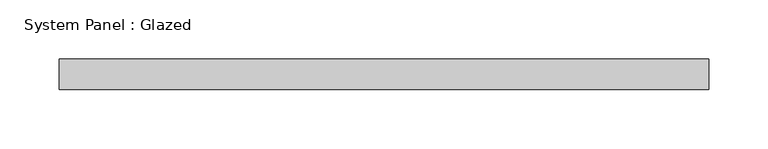
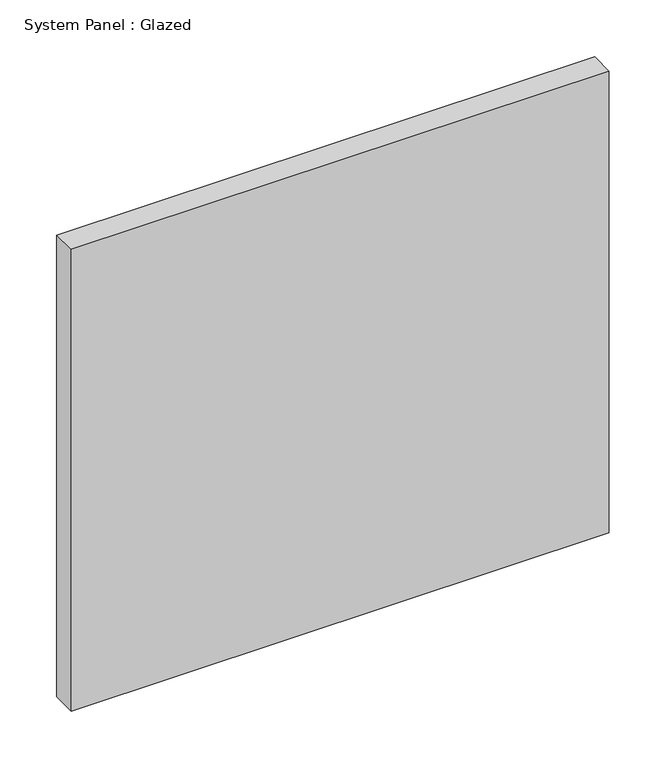
"""IFC4 building model written with IfcOpenShell, lengths in millimetres: plate geometry, System Panel : Glazed."""

from ifc_helpers import new_model, si_unit, origin, origin_with_axes, place, context, project, spatial, polyline, outline, extrude, source, transform, mapped, element, save


def system_panel_glazed_0f474f61(model_context):
    return source(origin(), model_context, "Body", "SweptSolid", [
        extrude(outline(polyline([(273.05, 19.05), (-273.05, 19.05), (-273.05, 44.45), (273.05, 44.45), (273.05, 19.05)])), origin_with_axes(), (0.0, 0.0, 1.0), 495.3),
    ])


if __name__ == "__main__":
    model = new_model("IFC4")
    model_context = context("Model", 3, world=origin())
    ifc_project = project(units=[si_unit("LENGTHUNIT", "METRE", prefix="MILLI")], contexts=[model_context])
    site = spatial("IfcSite", under=ifc_project)
    building = spatial("IfcBuilding", under=site)
    placement = place(None, origin())
    system_panel_glazed_shape = system_panel_glazed_0f474f61(model_context)
    element("IfcPlate", 1, ObjectType="System Panel : Glazed", at=placement, inside=building, context=model_context, shape_type="MappedRepresentation", body=[
        mapped(system_panel_glazed_shape, transform((0.0, 0.0, 0.0), x_axis=(1.0, 0.0, 0.0), y_axis=(0.0, 1.0, 0.0), z_axis=(0.0, 0.0, 1.0))),
    ])
    save(model, "model.ifc")

# Revit data of these elements
# Type "System Panel : Glazed"
#   Construction Type Id = "GSP4R"
#   Analytic Construction = "1/8 in Pilkington single glazing"
#   Visual Light Transmittance = 0.9
#   Solar Heat Gain Coefficient = 0.86
#   Heat Transfer Coefficient (U) = 1.18115 BTU/(h·ft²·°F)
#   Define Thermal Properties by = 1
# Element 1 (IfcPlate, "System Panel : Glazed")
#   Materials on its faces: "Glass"
# Materials
#   "Glass": class "Glass", colour RGB 0 128 192, transparency 0.75, Description = "Soda Lime Glass", Cost = 0
